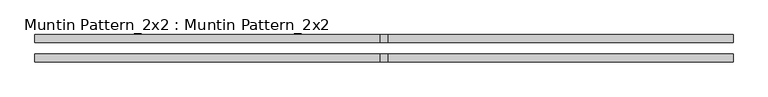
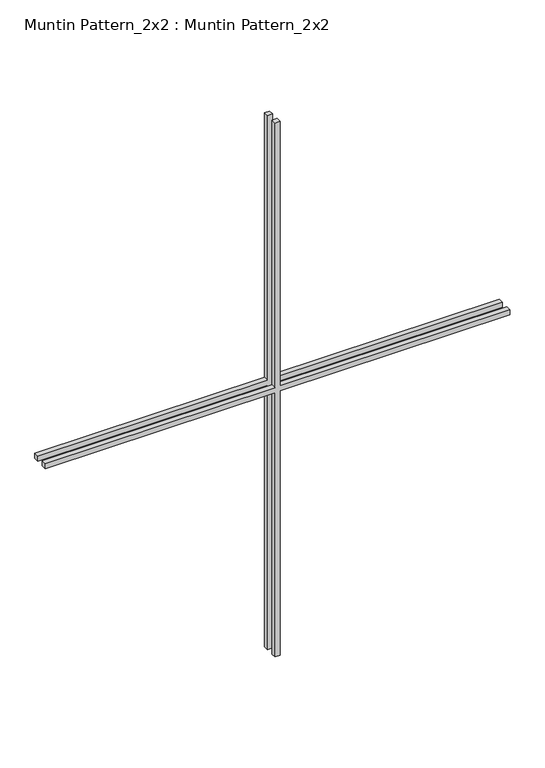
"""IFC4 building model written with IfcOpenShell, lengths in millimetres: proxy geometry, Muntin Pattern_2x2 : Muntin Pattern_2x2."""

from ifc_helpers import new_model, si_unit, frame, origin, place, context, project, spatial, polyline, outline, extrude, source, transform, mapped, element, save


def muntin_pattern_2x2_muntin_pattern_2x2_511ed329(model_context):
    return source(origin(), model_context, "Body", "SweptSolid", [
        extrude(outline(polyline([(698.5, -6.35), (698.5, -570.0914087), (685.8, -570.0914087), (685.8, -6.35), (0.0, -6.35), (0.0, 6.35), (685.8, 6.35), (685.8, 570.0914087), (698.5, 570.0914087), (698.5, 6.35), (1384.3, 6.35), (1384.3, -6.35), (698.5, -6.35)])), frame((0.0, 9.525, 0.0), z_axis=(0.0, 1.0, 0.0), x_axis=(0.0, 0.0, 1.0)), (0.0, 0.0, 1.0), 12.7),
        extrude(outline(polyline([(698.5, -6.35), (698.5, -570.0914087), (685.8, -570.0914087), (685.8, -6.35), (0.0, -6.35), (0.0, 6.35), (685.8, 6.35), (685.8, 570.0914087), (698.5, 570.0914087), (698.5, 6.35), (1384.3, 6.35), (1384.3, -6.35), (698.5, -6.35)])), frame((0.0, -22.225, 0.0), z_axis=(0.0, 1.0, 0.0), x_axis=(0.0, 0.0, 1.0)), (0.0, 0.0, 1.0), 12.7),
    ])


if __name__ == "__main__":
    model = new_model("IFC4")
    model_context = context("Model", 3, world=origin())
    ifc_project = project(units=[si_unit("LENGTHUNIT", "METRE", prefix="MILLI")], contexts=[model_context])
    site = spatial("IfcSite", under=ifc_project)
    building = spatial("IfcBuilding", under=site)
    placement = place(None, origin())
    muntin_pattern_2x2_muntin_pattern_2x2_shape = muntin_pattern_2x2_muntin_pattern_2x2_511ed329(model_context)
    element("IfcBuildingElementProxy", 1, Name="Muntin Pattern_2x2 : Muntin Pattern_2x2", ObjectType="Muntin Pattern_2x2 : Muntin Pattern_2x2", at=placement, inside=building, context=model_context, shape_type="MappedRepresentation", body=[
        mapped(muntin_pattern_2x2_muntin_pattern_2x2_shape, transform((0.0, 0.0, 0.0), x_axis=(1.0, 0.0, 0.0), y_axis=(0.0, 1.0, 0.0), z_axis=(0.0, 0.0, 1.0))),
    ])
    save(model, "model.ifc")

# Revit data of these elements
# Type "Muntin Pattern_2x2 : Muntin Pattern_2x2"
#   Width [instance default] = 4' - 0"
#   Thickness = 0' - 0 1/2"
#   Height [instance default] = 4' - 0"
#   Distance = 0' - 0 3/4"
#   Interior Material [instance default] = none
#   Exterior Material [instance default] = none
#   Default Elevation = 0
# Element 1 (IfcBuildingElementProxy, "Muntin Pattern_2x2 : Muntin Pattern_2x2")
#   Width = 3' - 8.88909"
#   Height = 4' - 6 1/2"
#   Interior Material = Wood - Stained
#   Exterior Material = Clad - White
#   Materials on its faces: "Clad - White", "Wood - Stained"
# Materials
#   "Clad - White": class "Wood", colour RGB 242 242 238, transparency 0, Cost = 0
#   "Wood - Stained": class "Wood", colour RGB 224 178 126, transparency 0, Cost = 0
